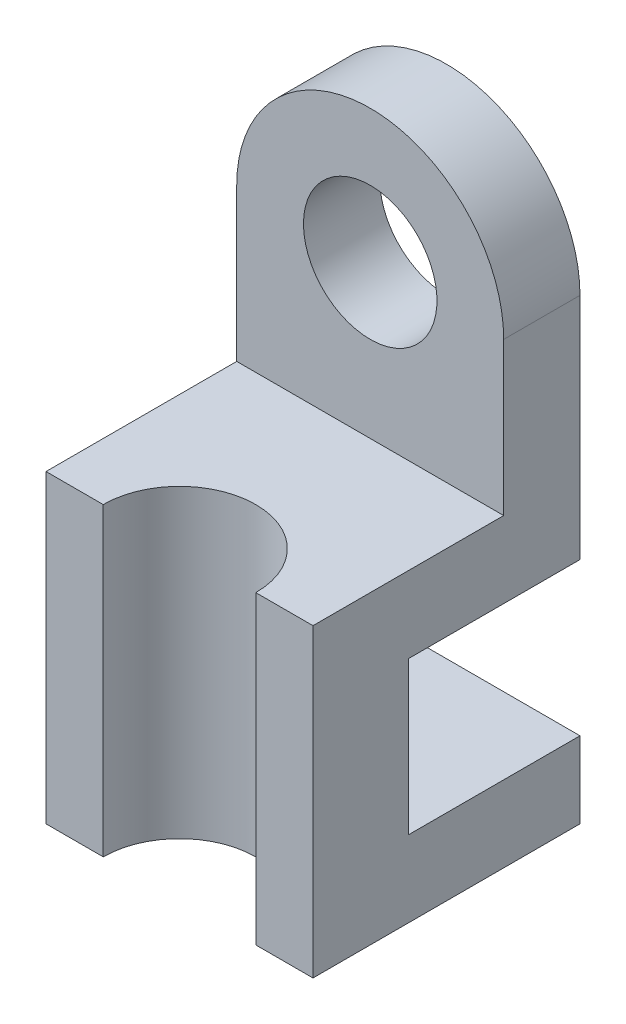
ISO-10303-21;
HEADER;
FILE_DESCRIPTION(('STEP AP214'),'2;1');
FILE_NAME('part.step','',(''),(''),'','','');
FILE_SCHEMA(('AUTOMOTIVE_DESIGN { 1 0 10303 214 1 1 1 1 }'));
ENDSEC;
DATA;
#1=APPLICATION_CONTEXT('core data for automotive mechanical design processes');
#2=APPLICATION_PROTOCOL_DEFINITION('international standard','automotive_design',2000,#1);
#3=PRODUCT_CONTEXT('',#1,'mechanical');
#4=PRODUCT('Part','Part','',(#3));
#5=PRODUCT_RELATED_PRODUCT_CATEGORY('part','',(#4));
#6=PRODUCT_DEFINITION_FORMATION('','',#4);
#7=PRODUCT_DEFINITION_CONTEXT('part definition',#1,'design');
#8=PRODUCT_DEFINITION('design','',#6,#7);
#9=PRODUCT_DEFINITION_SHAPE('','',#8);
#10=(LENGTH_UNIT() NAMED_UNIT(*) SI_UNIT(.MILLI.,.METRE.));
#11=(NAMED_UNIT(*) PLANE_ANGLE_UNIT() SI_UNIT($,.RADIAN.));
#12=(NAMED_UNIT(*) SI_UNIT($,.STERADIAN.) SOLID_ANGLE_UNIT());
#13=UNCERTAINTY_MEASURE_WITH_UNIT(LENGTH_MEASURE(1.E-05),#10,'distance_accuracy_value','');
#14=(GEOMETRIC_REPRESENTATION_CONTEXT(3) GLOBAL_UNCERTAINTY_ASSIGNED_CONTEXT((#13)) GLOBAL_UNIT_ASSIGNED_CONTEXT((#10,
#11,#12)) REPRESENTATION_CONTEXT('',''));
#15=CARTESIAN_POINT('',(0.,0.,0.));
#16=DIRECTION('',(0.,0.,1.));
#17=DIRECTION('',(1.,0.,0.));
#18=AXIS2_PLACEMENT_3D('',#15,#16,#17);
#19=CARTESIAN_POINT('',(0.,20.,35.));
#20=DIRECTION('',(0.,1.,0.));
#21=DIRECTION('',(0.,0.,1.));
#22=AXIS2_PLACEMENT_3D('',#19,#20,#21);
#23=PLANE('',#22);
#24=DIRECTION('',(0.,0.,-1.));
#25=VECTOR('',#24,1.);
#26=CARTESIAN_POINT('',(35.,20.,-35.));
#27=LINE('',#26,#25);
#28=CARTESIAN_POINT('',(35.,20.,35.));
#29=VERTEX_POINT('',#28);
#30=CARTESIAN_POINT('',(35.,20.,-15.));
#31=VERTEX_POINT('',#30);
#32=EDGE_CURVE('E207',#29,#31,#27,.T.);
#33=ORIENTED_EDGE('',*,*,#32,.T.);
#34=DIRECTION('',(-1.,0.,0.));
#35=VECTOR('',#34,1.);
#36=CARTESIAN_POINT('',(35.,20.,-15.));
#37=LINE('',#36,#35);
#38=CARTESIAN_POINT('',(-35.,20.,-15.));
#39=VERTEX_POINT('',#38);
#40=EDGE_CURVE('E156',#31,#39,#37,.T.);
#41=ORIENTED_EDGE('',*,*,#40,.T.);
#42=DIRECTION('',(0.,0.,1.));
#43=VECTOR('',#42,1.);
#44=CARTESIAN_POINT('',(-35.,20.,-35.));
#45=LINE('',#44,#43);
#46=CARTESIAN_POINT('',(-35.,20.,35.));
#47=VERTEX_POINT('',#46);
#48=EDGE_CURVE('E93',#39,#47,#45,.T.);
#49=ORIENTED_EDGE('',*,*,#48,.T.);
#50=DIRECTION('',(1.,0.,0.));
#51=VECTOR('',#50,1.);
#52=CARTESIAN_POINT('',(-35.,20.,35.));
#53=LINE('',#52,#51);
#54=CARTESIAN_POINT('',(-20.,20.,35.));
#55=VERTEX_POINT('',#54);
#56=EDGE_CURVE('E213',#47,#55,#53,.T.);
#57=ORIENTED_EDGE('',*,*,#56,.T.);
#58=CARTESIAN_POINT('',(0.,20.,35.));
#59=DIRECTION('',(0.,-1.,0.));
#60=DIRECTION('',(0.,0.,1.));
#61=AXIS2_PLACEMENT_3D('',#58,#59,#60);
#62=CIRCLE('',#61,20.);
#63=CARTESIAN_POINT('',(20.,20.,35.));
#64=VERTEX_POINT('',#63);
#65=EDGE_CURVE('E214',#55,#64,#62,.T.);
#66=ORIENTED_EDGE('',*,*,#65,.T.);
#67=DIRECTION('',(1.,0.,0.));
#68=VECTOR('',#67,1.);
#69=CARTESIAN_POINT('',(20.,20.,35.));
#70=LINE('',#69,#68);
#71=EDGE_CURVE('E69',#64,#29,#70,.T.);
#72=ORIENTED_EDGE('',*,*,#71,.T.);
#73=EDGE_LOOP('',(#33,#41,#49,#57,#66,#72));
#74=FACE_BOUND('',#73,.T.);
#75=ADVANCED_FACE('F44',(#74),#23,.T.);
#76=CARTESIAN_POINT('',(35.,20.,-35.));
#77=DIRECTION('',(-1.,0.,0.));
#78=DIRECTION('',(0.,0.,1.));
#79=AXIS2_PLACEMENT_3D('',#76,#77,#78);
#80=PLANE('',#79);
#81=DIRECTION('',(0.,-1.,0.));
#82=VECTOR('',#81,1.);
#83=CARTESIAN_POINT('',(35.,20.,-35.));
#84=LINE('',#83,#82);
#85=CARTESIAN_POINT('',(35.,60.,-35.));
#86=VERTEX_POINT('',#85);
#87=CARTESIAN_POINT('',(35.,0.,-35.));
#88=VERTEX_POINT('',#87);
#89=EDGE_CURVE('E52',#86,#88,#84,.T.);
#90=ORIENTED_EDGE('',*,*,#89,.F.);
#91=DIRECTION('',(0.,0.,-1.));
#92=VECTOR('',#91,1.);
#93=CARTESIAN_POINT('',(35.,60.,-15.));
#94=LINE('',#93,#92);
#95=CARTESIAN_POINT('',(35.,60.,-15.));
#96=VERTEX_POINT('',#95);
#97=EDGE_CURVE('E145',#96,#86,#94,.T.);
#98=ORIENTED_EDGE('',*,*,#97,.F.);
#99=DIRECTION('',(0.,-1.,0.));
#100=VECTOR('',#99,1.);
#101=CARTESIAN_POINT('',(35.,60.,-15.));
#102=LINE('',#101,#100);
#103=EDGE_CURVE('E150',#96,#31,#102,.T.);
#104=ORIENTED_EDGE('',*,*,#103,.T.);
#105=ORIENTED_EDGE('',*,*,#32,.F.);
#106=DIRECTION('',(0.,-1.,0.));
#107=VECTOR('',#106,1.);
#108=CARTESIAN_POINT('',(35.,20.,35.));
#109=LINE('',#108,#107);
#110=CARTESIAN_POINT('',(35.,-60.,35.));
#111=VERTEX_POINT('',#110);
#112=EDGE_CURVE('E217',#29,#111,#109,.T.);
#113=ORIENTED_EDGE('',*,*,#112,.T.);
#114=DIRECTION('',(0.,0.,1.));
#115=VECTOR('',#114,1.);
#116=CARTESIAN_POINT('',(35.,-60.,35.));
#117=LINE('',#116,#115);
#118=CARTESIAN_POINT('',(35.,-60.,-35.));
#119=VERTEX_POINT('',#118);
#120=EDGE_CURVE('E179',#119,#111,#117,.T.);
#121=ORIENTED_EDGE('',*,*,#120,.F.);
#122=DIRECTION('',(0.,1.,0.));
#123=VECTOR('',#122,1.);
#124=CARTESIAN_POINT('',(35.,-60.,-35.));
#125=LINE('',#124,#123);
#126=CARTESIAN_POINT('',(35.,-40.,-35.));
#127=VERTEX_POINT('',#126);
#128=EDGE_CURVE('E188',#119,#127,#125,.T.);
#129=ORIENTED_EDGE('',*,*,#128,.T.);
#130=DIRECTION('',(0.,0.,1.));
#131=VECTOR('',#130,1.);
#132=CARTESIAN_POINT('',(35.,-40.,35.));
#133=LINE('',#132,#131);
#134=CARTESIAN_POINT('',(35.,-40.,10.));
#135=VERTEX_POINT('',#134);
#136=EDGE_CURVE('E168',#127,#135,#133,.T.);
#137=ORIENTED_EDGE('',*,*,#136,.T.);
#138=DIRECTION('',(0.,1.,0.));
#139=VECTOR('',#138,1.);
#140=CARTESIAN_POINT('',(35.,-40.,10.));
#141=LINE('',#140,#139);
#142=CARTESIAN_POINT('',(35.,0.,10.));
#143=VERTEX_POINT('',#142);
#144=EDGE_CURVE('E201',#135,#143,#141,.T.);
#145=ORIENTED_EDGE('',*,*,#144,.T.);
#146=DIRECTION('',(0.,0.,-1.));
#147=VECTOR('',#146,1.);
#148=CARTESIAN_POINT('',(35.,0.,-35.));
#149=LINE('',#148,#147);
#150=EDGE_CURVE('E206',#143,#88,#149,.T.);
#151=ORIENTED_EDGE('',*,*,#150,.T.);
#152=EDGE_LOOP('',(#90,#98,#104,#105,#113,#121,#129,#137,#145,#151));
#153=FACE_BOUND('',#152,.T.);
#154=ADVANCED_FACE('F50',(#153),#80,.F.);
#155=CARTESIAN_POINT('',(-35.,20.,-35.));
#156=DIRECTION('',(0.,0.,1.));
#157=DIRECTION('',(1.,0.,0.));
#158=AXIS2_PLACEMENT_3D('',#155,#156,#157);
#159=PLANE('',#158);
#160=DIRECTION('',(-1.,0.,0.));
#161=VECTOR('',#160,1.);
#162=CARTESIAN_POINT('',(-35.,0.,-35.));
#163=LINE('',#162,#161);
#164=CARTESIAN_POINT('',(-35.,0.,-35.));
#165=VERTEX_POINT('',#164);
#166=EDGE_CURVE('E82',#88,#165,#163,.T.);
#167=ORIENTED_EDGE('',*,*,#166,.T.);
#168=DIRECTION('',(0.,-1.,0.));
#169=VECTOR('',#168,1.);
#170=CARTESIAN_POINT('',(-35.,20.,-35.));
#171=LINE('',#170,#169);
#172=CARTESIAN_POINT('',(-35.,60.,-35.));
#173=VERTEX_POINT('',#172);
#174=EDGE_CURVE('E227',#173,#165,#171,.T.);
#175=ORIENTED_EDGE('',*,*,#174,.F.);
#176=CARTESIAN_POINT('',(0.,60.,-35.));
#177=DIRECTION('',(0.,0.,-1.));
#178=DIRECTION('',(-1.,0.,0.));
#179=AXIS2_PLACEMENT_3D('',#176,#177,#178);
#180=CIRCLE('',#179,35.);
#181=EDGE_CURVE('E159',#173,#86,#180,.T.);
#182=ORIENTED_EDGE('',*,*,#181,.T.);
#183=ORIENTED_EDGE('',*,*,#89,.T.);
#184=EDGE_LOOP('',(#167,#175,#182,#183));
#185=FACE_BOUND('',#184,.T.);
#186=CARTESIAN_POINT('',(0.,60.,-35.));
#187=DIRECTION('',(0.,0.,-1.));
#188=DIRECTION('',(-1.,0.,0.));
#189=AXIS2_PLACEMENT_3D('',#186,#187,#188);
#190=CIRCLE('',#189,17.5);
#191=CARTESIAN_POINT('',(-17.5,60.,-35.));
#192=VERTEX_POINT('',#191);
#193=EDGE_CURVE('E164',#192,#192,#190,.T.);
#194=ORIENTED_EDGE('',*,*,#193,.F.);
#195=EDGE_LOOP('',(#194));
#196=FACE_BOUND('',#195,.T.);
#197=ADVANCED_FACE('F233',(#185,#196),#159,.F.);
#198=CARTESIAN_POINT('',(-35.,20.,-35.));
#199=DIRECTION('',(1.,0.,0.));
#200=DIRECTION('',(0.,0.,-1.));
#201=AXIS2_PLACEMENT_3D('',#198,#199,#200);
#202=PLANE('',#201);
#203=DIRECTION('',(0.,0.,1.));
#204=VECTOR('',#203,1.);
#205=CARTESIAN_POINT('',(-35.,0.,-35.));
#206=LINE('',#205,#204);
#207=CARTESIAN_POINT('',(-35.,0.,10.));
#208=VERTEX_POINT('',#207);
#209=EDGE_CURVE('E211',#165,#208,#206,.T.);
#210=ORIENTED_EDGE('',*,*,#209,.T.);
#211=DIRECTION('',(0.,1.,0.));
#212=VECTOR('',#211,1.);
#213=CARTESIAN_POINT('',(-35.,-40.,10.));
#214=LINE('',#213,#212);
#215=CARTESIAN_POINT('',(-35.,-40.,10.));
#216=VERTEX_POINT('',#215);
#217=EDGE_CURVE('E204',#216,#208,#214,.T.);
#218=ORIENTED_EDGE('',*,*,#217,.F.);
#219=DIRECTION('',(0.,0.,-1.));
#220=VECTOR('',#219,1.);
#221=CARTESIAN_POINT('',(-35.,-40.,35.));
#222=LINE('',#221,#220);
#223=CARTESIAN_POINT('',(-35.,-40.,-35.));
#224=VERTEX_POINT('',#223);
#225=EDGE_CURVE('E178',#216,#224,#222,.T.);
#226=ORIENTED_EDGE('',*,*,#225,.T.);
#227=DIRECTION('',(0.,1.,0.));
#228=VECTOR('',#227,1.);
#229=CARTESIAN_POINT('',(-35.,-60.,-35.));
#230=LINE('',#229,#228);
#231=CARTESIAN_POINT('',(-35.,-60.,-35.));
#232=VERTEX_POINT('',#231);
#233=EDGE_CURVE('E192',#232,#224,#230,.T.);
#234=ORIENTED_EDGE('',*,*,#233,.F.);
#235=DIRECTION('',(0.,0.,-1.));
#236=VECTOR('',#235,1.);
#237=CARTESIAN_POINT('',(-35.,-60.,35.));
#238=LINE('',#237,#236);
#239=CARTESIAN_POINT('',(-35.,-60.,35.));
#240=VERTEX_POINT('',#239);
#241=EDGE_CURVE('E184',#240,#232,#238,.T.);
#242=ORIENTED_EDGE('',*,*,#241,.F.);
#243=DIRECTION('',(0.,-1.,0.));
#244=VECTOR('',#243,1.);
#245=CARTESIAN_POINT('',(-35.,20.,35.));
#246=LINE('',#245,#244);
#247=EDGE_CURVE('E230',#47,#240,#246,.T.);
#248=ORIENTED_EDGE('',*,*,#247,.F.);
#249=ORIENTED_EDGE('',*,*,#48,.F.);
#250=DIRECTION('',(0.,1.,0.));
#251=VECTOR('',#250,1.);
#252=CARTESIAN_POINT('',(-35.,20.,-15.));
#253=LINE('',#252,#251);
#254=CARTESIAN_POINT('',(-35.,60.,-15.));
#255=VERTEX_POINT('',#254);
#256=EDGE_CURVE('E58',#39,#255,#253,.T.);
#257=ORIENTED_EDGE('',*,*,#256,.T.);
#258=DIRECTION('',(0.,0.,-1.));
#259=VECTOR('',#258,1.);
#260=CARTESIAN_POINT('',(-35.,60.,-15.));
#261=LINE('',#260,#259);
#262=EDGE_CURVE('E155',#255,#173,#261,.T.);
#263=ORIENTED_EDGE('',*,*,#262,.T.);
#264=ORIENTED_EDGE('',*,*,#174,.T.);
#265=EDGE_LOOP('',(#210,#218,#226,#234,#242,#248,#249,#257,#263,#264));
#266=FACE_BOUND('',#265,.T.);
#267=ADVANCED_FACE('F232',(#266),#202,.F.);
#268=CARTESIAN_POINT('',(-35.,20.,35.));
#269=DIRECTION('',(0.,0.,-1.));
#270=DIRECTION('',(-1.,0.,0.));
#271=AXIS2_PLACEMENT_3D('',#268,#269,#270);
#272=PLANE('',#271);
#273=ORIENTED_EDGE('',*,*,#247,.T.);
#274=DIRECTION('',(-1.,0.,0.));
#275=VECTOR('',#274,1.);
#276=CARTESIAN_POINT('',(0.,-60.,35.));
#277=LINE('',#276,#275);
#278=CARTESIAN_POINT('',(-20.,-60.,35.));
#279=VERTEX_POINT('',#278);
#280=EDGE_CURVE('E189',#279,#240,#277,.T.);
#281=ORIENTED_EDGE('',*,*,#280,.F.);
#282=DIRECTION('',(0.,-1.,0.));
#283=VECTOR('',#282,1.);
#284=CARTESIAN_POINT('',(-20.,20.,35.));
#285=LINE('',#284,#283);
#286=EDGE_CURVE('E229',#55,#279,#285,.T.);
#287=ORIENTED_EDGE('',*,*,#286,.F.);
#288=ORIENTED_EDGE('',*,*,#56,.F.);
#289=EDGE_LOOP('',(#273,#281,#287,#288));
#290=FACE_BOUND('',#289,.T.);
#291=ADVANCED_FACE('F241',(#290),#272,.F.);
#292=CARTESIAN_POINT('',(0.,20.,35.));
#293=DIRECTION('',(0.,-1.,0.));
#294=DIRECTION('',(0.,0.,-1.));
#295=AXIS2_PLACEMENT_3D('',#292,#293,#294);
#296=CYLINDRICAL_SURFACE('',#295,20.);
#297=ORIENTED_EDGE('',*,*,#286,.T.);
#298=CARTESIAN_POINT('',(0.,-60.,35.));
#299=DIRECTION('',(0.,-1.,0.));
#300=DIRECTION('',(0.,0.,-1.));
#301=AXIS2_PLACEMENT_3D('',#298,#299,#300);
#302=CIRCLE('',#301,20.);
#303=CARTESIAN_POINT('',(20.,-60.,35.));
#304=VERTEX_POINT('',#303);
#305=EDGE_CURVE('E171',#279,#304,#302,.T.);
#306=ORIENTED_EDGE('',*,*,#305,.T.);
#307=DIRECTION('',(0.,-1.,0.));
#308=VECTOR('',#307,1.);
#309=CARTESIAN_POINT('',(20.,20.,35.));
#310=LINE('',#309,#308);
#311=EDGE_CURVE('E221',#64,#304,#310,.T.);
#312=ORIENTED_EDGE('',*,*,#311,.F.);
#313=ORIENTED_EDGE('',*,*,#65,.F.);
#314=EDGE_LOOP('',(#297,#306,#312,#313));
#315=FACE_BOUND('',#314,.T.);
#316=ADVANCED_FACE('F248',(#315),#296,.F.);
#317=CARTESIAN_POINT('',(20.,20.,35.));
#318=DIRECTION('',(0.,0.,-1.));
#319=DIRECTION('',(-1.,0.,0.));
#320=AXIS2_PLACEMENT_3D('',#317,#318,#319);
#321=PLANE('',#320);
#322=ORIENTED_EDGE('',*,*,#311,.T.);
#323=DIRECTION('',(-1.,0.,0.));
#324=VECTOR('',#323,1.);
#325=CARTESIAN_POINT('',(0.,-60.,35.));
#326=LINE('',#325,#324);
#327=EDGE_CURVE('E172',#111,#304,#326,.T.);
#328=ORIENTED_EDGE('',*,*,#327,.F.);
#329=ORIENTED_EDGE('',*,*,#112,.F.);
#330=ORIENTED_EDGE('',*,*,#71,.F.);
#331=EDGE_LOOP('',(#322,#328,#329,#330));
#332=FACE_BOUND('',#331,.T.);
#333=ADVANCED_FACE('F247',(#332),#321,.F.);
#334=CARTESIAN_POINT('',(0.,0.,35.));
#335=DIRECTION('',(0.,1.,0.));
#336=DIRECTION('',(0.,0.,1.));
#337=AXIS2_PLACEMENT_3D('',#334,#335,#336);
#338=PLANE('',#337);
#339=ORIENTED_EDGE('',*,*,#150,.F.);
#340=DIRECTION('',(-1.,0.,0.));
#341=VECTOR('',#340,1.);
#342=CARTESIAN_POINT('',(0.,0.,10.));
#343=LINE('',#342,#341);
#344=EDGE_CURVE('E11',#143,#208,#343,.T.);
#345=ORIENTED_EDGE('',*,*,#344,.T.);
#346=ORIENTED_EDGE('',*,*,#209,.F.);
#347=ORIENTED_EDGE('',*,*,#166,.F.);
#348=EDGE_LOOP('',(#339,#345,#346,#347));
#349=FACE_BOUND('',#348,.T.);
#350=ADVANCED_FACE('F268',(#349),#338,.F.);
#351=CARTESIAN_POINT('',(35.,-40.,10.));
#352=DIRECTION('',(0.,0.,-1.));
#353=DIRECTION('',(-1.,0.,0.));
#354=AXIS2_PLACEMENT_3D('',#351,#352,#353);
#355=PLANE('',#354);
#356=ORIENTED_EDGE('',*,*,#344,.F.);
#357=ORIENTED_EDGE('',*,*,#144,.F.);
#358=DIRECTION('',(-1.,0.,0.));
#359=VECTOR('',#358,1.);
#360=CARTESIAN_POINT('',(35.,-40.,10.));
#361=LINE('',#360,#359);
#362=EDGE_CURVE('E196',#135,#216,#361,.T.);
#363=ORIENTED_EDGE('',*,*,#362,.T.);
#364=ORIENTED_EDGE('',*,*,#217,.T.);
#365=EDGE_LOOP('',(#356,#357,#363,#364));
#366=FACE_BOUND('',#365,.T.);
#367=ADVANCED_FACE('F264',(#366),#355,.T.);
#368=CARTESIAN_POINT('',(0.,-60.,-35.));
#369=DIRECTION('',(0.,0.,1.));
#370=DIRECTION('',(1.,0.,0.));
#371=AXIS2_PLACEMENT_3D('',#368,#369,#370);
#372=PLANE('',#371);
#373=DIRECTION('',(1.,0.,0.));
#374=VECTOR('',#373,1.);
#375=CARTESIAN_POINT('',(0.,-40.,-35.));
#376=LINE('',#375,#374);
#377=EDGE_CURVE('E195',#224,#127,#376,.T.);
#378=ORIENTED_EDGE('',*,*,#377,.T.);
#379=ORIENTED_EDGE('',*,*,#128,.F.);
#380=DIRECTION('',(1.,0.,0.));
#381=VECTOR('',#380,1.);
#382=CARTESIAN_POINT('',(0.,-60.,-35.));
#383=LINE('',#382,#381);
#384=EDGE_CURVE('E185',#232,#119,#383,.T.);
#385=ORIENTED_EDGE('',*,*,#384,.F.);
#386=ORIENTED_EDGE('',*,*,#233,.T.);
#387=EDGE_LOOP('',(#378,#379,#385,#386));
#388=FACE_BOUND('',#387,.T.);
#389=ADVANCED_FACE('F260',(#388),#372,.F.);
#390=CARTESIAN_POINT('',(0.,-60.,35.));
#391=DIRECTION('',(0.,-1.,0.));
#392=DIRECTION('',(0.,0.,-1.));
#393=AXIS2_PLACEMENT_3D('',#390,#391,#392);
#394=PLANE('',#393);
#395=ORIENTED_EDGE('',*,*,#305,.F.);
#396=ORIENTED_EDGE('',*,*,#280,.T.);
#397=ORIENTED_EDGE('',*,*,#241,.T.);
#398=ORIENTED_EDGE('',*,*,#384,.T.);
#399=ORIENTED_EDGE('',*,*,#120,.T.);
#400=ORIENTED_EDGE('',*,*,#327,.T.);
#401=EDGE_LOOP('',(#395,#396,#397,#398,#399,#400));
#402=FACE_BOUND('',#401,.T.);
#403=ADVANCED_FACE('F251',(#402),#394,.T.);
#404=CARTESIAN_POINT('',(0.,-40.,35.));
#405=DIRECTION('',(0.,-1.,0.));
#406=DIRECTION('',(0.,0.,-1.));
#407=AXIS2_PLACEMENT_3D('',#404,#405,#406);
#408=PLANE('',#407);
#409=ORIENTED_EDGE('',*,*,#362,.F.);
#410=ORIENTED_EDGE('',*,*,#136,.F.);
#411=ORIENTED_EDGE('',*,*,#377,.F.);
#412=ORIENTED_EDGE('',*,*,#225,.F.);
#413=EDGE_LOOP('',(#409,#410,#411,#412));
#414=FACE_BOUND('',#413,.T.);
#415=ADVANCED_FACE('F265',(#414),#408,.F.);
#416=CARTESIAN_POINT('',(0.,60.,-15.));
#417=DIRECTION('',(0.,0.,-1.));
#418=DIRECTION('',(-1.,0.,0.));
#419=AXIS2_PLACEMENT_3D('',#416,#417,#418);
#420=CYLINDRICAL_SURFACE('',#419,35.);
#421=ORIENTED_EDGE('',*,*,#181,.F.);
#422=ORIENTED_EDGE('',*,*,#262,.F.);
#423=CARTESIAN_POINT('',(0.,60.,-15.));
#424=DIRECTION('',(0.,0.,-1.));
#425=DIRECTION('',(-1.,0.,0.));
#426=AXIS2_PLACEMENT_3D('',#423,#424,#425);
#427=CIRCLE('',#426,35.);
#428=EDGE_CURVE('E154',#255,#96,#427,.T.);
#429=ORIENTED_EDGE('',*,*,#428,.T.);
#430=ORIENTED_EDGE('',*,*,#97,.T.);
#431=EDGE_LOOP('',(#421,#422,#429,#430));
#432=FACE_BOUND('',#431,.T.);
#433=ADVANCED_FACE('F158',(#432),#420,.T.);
#434=CARTESIAN_POINT('',(0.,60.,-15.));
#435=DIRECTION('',(0.,0.,-1.));
#436=DIRECTION('',(-1.,0.,0.));
#437=AXIS2_PLACEMENT_3D('',#434,#435,#436);
#438=PLANE('',#437);
#439=CARTESIAN_POINT('',(0.,60.,-15.));
#440=DIRECTION('',(0.,0.,-1.));
#441=DIRECTION('',(-1.,0.,0.));
#442=AXIS2_PLACEMENT_3D('',#439,#440,#441);
#443=CIRCLE('',#442,17.5);
#444=CARTESIAN_POINT('',(-17.5,60.,-15.));
#445=VERTEX_POINT('',#444);
#446=EDGE_CURVE('E165',#445,#445,#443,.T.);
#447=ORIENTED_EDGE('',*,*,#446,.T.);
#448=EDGE_LOOP('',(#447));
#449=FACE_BOUND('',#448,.T.);
#450=ORIENTED_EDGE('',*,*,#428,.F.);
#451=ORIENTED_EDGE('',*,*,#256,.F.);
#452=ORIENTED_EDGE('',*,*,#40,.F.);
#453=ORIENTED_EDGE('',*,*,#103,.F.);
#454=EDGE_LOOP('',(#450,#451,#452,#453));
#455=FACE_BOUND('',#454,.T.);
#456=ADVANCED_FACE('F152',(#449,#455),#438,.F.);
#457=CARTESIAN_POINT('',(0.,60.,-15.));
#458=DIRECTION('',(0.,0.,-1.));
#459=DIRECTION('',(-1.,0.,0.));
#460=AXIS2_PLACEMENT_3D('',#457,#458,#459);
#461=CYLINDRICAL_SURFACE('',#460,17.5);
#462=ORIENTED_EDGE('',*,*,#446,.F.);
#463=EDGE_LOOP('',(#462));
#464=FACE_BOUND('',#463,.T.);
#465=ORIENTED_EDGE('',*,*,#193,.T.);
#466=EDGE_LOOP('',(#465));
#467=FACE_BOUND('',#466,.T.);
#468=ADVANCED_FACE('F294',(#464,#467),#461,.F.);
#469=CLOSED_SHELL('',(#75,#154,#197,#267,#291,#316,#333,#350,#367,#389,#403,#415,#433,#456,#468));
#470=MANIFOLD_SOLID_BREP('B2',#469);
#471=ADVANCED_BREP_SHAPE_REPRESENTATION('',(#18,#470),#14);
#472=SHAPE_DEFINITION_REPRESENTATION(#9,#471);
ENDSEC;
END-ISO-10303-21;
